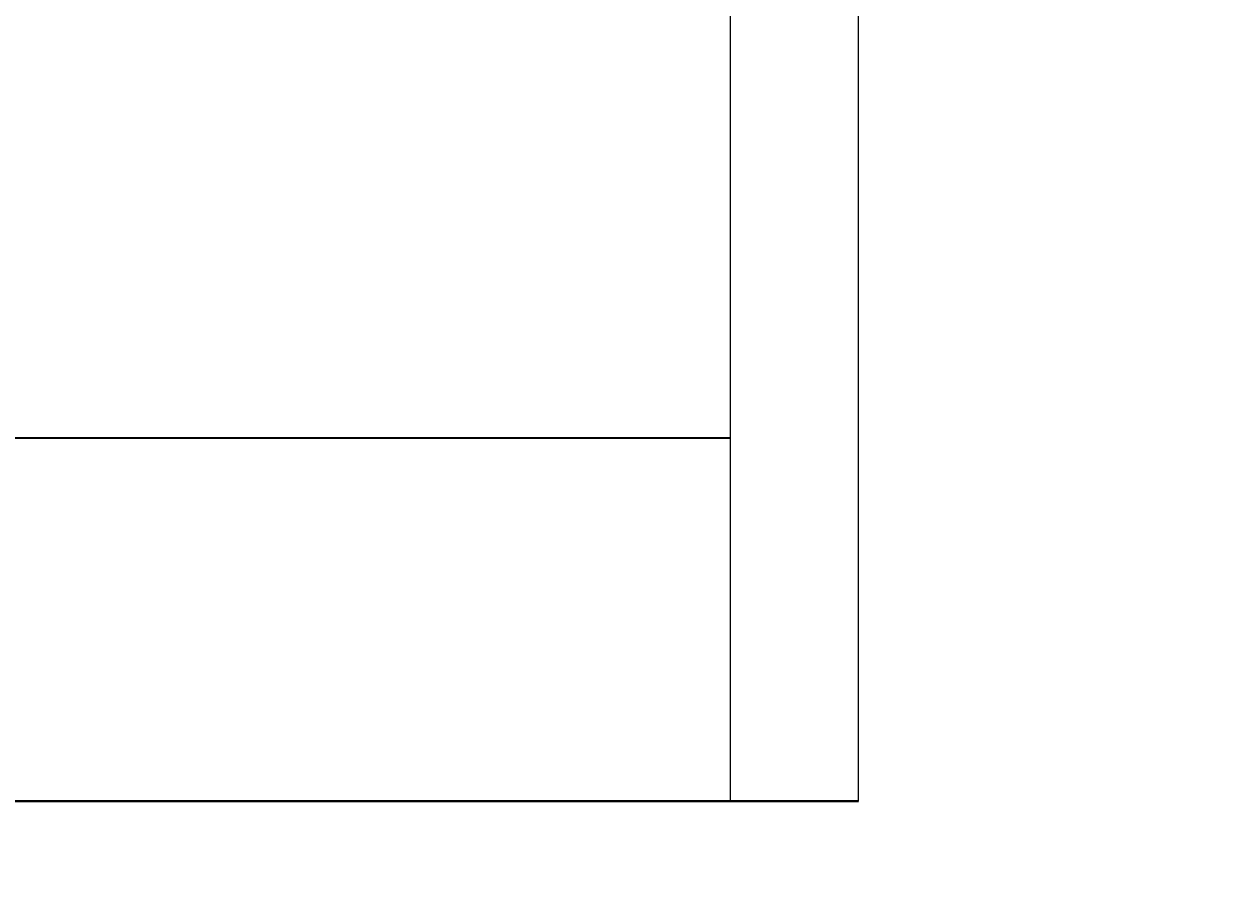
# Model space of a CAD drawing. Units: millimetres. Extents: x 19292 to 100733, y 12374 to 26974.
# Tile 5 of 24: x 29028 to 29777, y 14845 to 15391. Entities that reach past the tile are written whole.
import ezdxf

# ---------------------------------------------------------------- set-up
doc = ezdxf.new("R2010")
doc.units = ezdxf.units.MM
for name, color, linetype, lineweight in [('A-ANNO-DIMS', 2, 'Continuous', 18), ('A-DOOR', 4, 'Continuous', 25), ('A-FLOR-PATT', 252, 'Continuous', 13), ('A-WALL', 7, 'Continuous', 35)]:
    doc.layers.add(name, color=color, linetype=linetype, lineweight=lineweight)
doc.styles.get("Standard").update_dxf_attribs({"font": 'arial.ttf'})
doc.dimstyles.get("Standard").update_dxf_attribs({"dimtxt": 0.18, "dimasz": 0.18, "dimexe": 0.18, "dimexo": 0.0625, "dimgap": 0.09, "dimtad": 0, "dimtih": 1, "dimtoh": 1, "dimdec": 4, "dimzin": 0, "dimdsep": 46, "dimtxsty": 'Standard', "dimcen": 0.09, "dimadec": 0, "dimazin": 0, "dimtfac": 1, "dimtdec": 4, "dimtofl": 0, "dimtmove": 0, "dimatfit": 3, "dimfxl": 1, "dimtolj": 1, "dimtzin": 0, "dimarcsym": 0})

# ---------------------------------------------------------------- blocks, each defined once
blk = doc.blocks.new('*D79')
at = {"layer": 'A-ANNO-DIMS', "color": 0, "lineweight": -2, "transparency": 16777216}
for p, q in [((22694.13, 22860.66), (22694.13, 12808.81)), ((36144.17, 15985.66), (36144.17, 12808.81)), ((22694.31, 12808.99), (29418.73, 12808.99)), ((36143.99, 12808.99), (29419.57, 12808.99))]:
    blk.add_line(p, q, dxfattribs=at)
at = {"layer": 'A-ANNO-DIMS', "color": 0, "transparency": 16777216}
for points in [[(22694.31, 12809.02), (22694.31, 12808.96), (22694.13, 12808.99)], [(36143.99, 12809.02), (36143.99, 12808.96), (36144.17, 12808.99)]]:
    blk.add_solid(points, dxfattribs=at)
at = {"layer": 'Defpoints', "color": 0, "transparency": 16777216}
for p in [(22694.13, 22860.72), (36144.17, 15985.72), (36144.17, 12808.99)]:
    blk.add_point(p, dxfattribs=at)
at = {"layer": 'A-ANNO-DIMS', "color": 0, "transparency": 16777216, "insert": (29419.15, 12808.99), "char_height": 0.18, "attachment_point": 5}
blk.add_mtext('\\A1;13450', dxfattribs=at)
blk = doc.blocks.new('*D82')
at = {"layer": 'A-ANNO-DIMS', "color": 0, "lineweight": -2, "transparency": 16777216}
for p, q in [((27198.81, 13562.81), (27198.81, 23555.9)), ((27198.99, 23555.72), (29296.44, 23555.72)), ((31394.62, 23555.72), (29297.17, 23555.72)), ((31394.8, 13544.06), (31394.8, 23555.9))]:
    blk.add_line(p, q, dxfattribs=at)
at = {"layer": 'A-ANNO-DIMS', "color": 0, "transparency": 16777216}
for points in [[(27198.99, 23555.75), (27198.99, 23555.69), (27198.81, 23555.72)], [(31394.62, 23555.75), (31394.62, 23555.69), (31394.8, 23555.72)]]:
    blk.add_solid(points, dxfattribs=at)
at = {"layer": 'Defpoints', "color": 0, "transparency": 16777216}
for p in [(31394.8, 23555.72), (27198.81, 13562.75), (31394.8, 13543.99)]:
    blk.add_point(p, dxfattribs=at)
at = {"layer": 'A-ANNO-DIMS', "color": 0, "transparency": 16777216, "insert": (29296.81, 23555.72), "char_height": 0.18, "attachment_point": 5}
blk.add_mtext('\\A1;4196', dxfattribs=at)
blk = doc.blocks.new('*D86')
at = {"layer": 'A-ANNO-DIMS', "color": 0, "lineweight": -2, "transparency": 16777216}
for p, q in [((27198.81, 15132.81), (27198.81, 23555.9)), ((27198.99, 23555.72), (29198.45, 23555.72)), ((31198.63, 23555.72), (29199.18, 23555.72)), ((31198.81, 15132.81), (31198.81, 23555.9))]:
    blk.add_line(p, q, dxfattribs=at)
at = {"layer": 'A-ANNO-DIMS', "color": 0, "transparency": 16777216}
for points in [[(27198.99, 23555.75), (27198.99, 23555.69), (27198.81, 23555.72)], [(31198.63, 23555.75), (31198.63, 23555.69), (31198.81, 23555.72)]]:
    blk.add_solid(points, dxfattribs=at)
at = {"layer": 'Defpoints', "color": 0, "transparency": 16777216}
for p in [(31198.81, 23555.72), (27198.81, 15132.75), (31198.81, 15132.75)]:
    blk.add_point(p, dxfattribs=at)
at = {"layer": 'A-ANNO-DIMS', "color": 0, "transparency": 16777216, "insert": (29198.81, 23555.72), "char_height": 0.18, "attachment_point": 5}
blk.add_mtext('\\A1;4000', dxfattribs=at)

msp = doc.modelspace()

# ---------------------------------------------------------------- hatches: boundary and pattern name
at = {"layer": 'A-FLOR-PATT'}
h = msp.add_hatch(dxfattribs=at)
h.set_pattern_fill('CROSS', color=256, scale=40)
h.paths.add_polyline_path([(31394.799, 14906.403), (31051.542, 14906.403), (29468.571, 14906.403), (27198.815, 14906.403), (27198.815, 13543.993), (31394.799, 13543.993)])
h.paths.add_polyline_path([(27828.096, 14036.581), (30629.164, 14036.581), (30629.164, 14443.478), (27828.096, 14443.478)], flags=24)

# ---------------------------------------------------------------- linework, layer by layer
at = {"layer": 'A-DOOR'}
for p, q in [((29468.571, 14906.403), (29468.571, 15641.675)), ((29548.571, 14906.403), (29548.571, 15641.675)), ((29468.571, 14906.403), (29548.571, 14906.403)), ((29468.571, 14906.403), (29548.571, 14906.403))]:
    msp.add_line(p, q, dxfattribs=at)
msp.add_arc((29468.571, 14906.403), 735.272, 0, 90, dxfattribs=at)
at = {"layer": 'A-WALL'}
for points in [[(29548.571, 14906.403), (27198.815, 14906.403), (27198.815, 13562.748), (23348.815, 13562.748), (23348.815, 19010.725), (22694.132, 19010.725), (22694.132, 22860.725), (28369.132, 22860.725), (28369.132, 21460.725), (31169.132, 21460.725), (31169.132, 22460.725), (34419.132, 22460.725), (34419.132, 22208.026)], [(29468.571, 15132.748), (27198.815, 15132.748), (27198.815, 17812.748)], [(31051.542, 14906.403), (31394.799, 14906.403), (31394.799, 13543.993), (27198.815, 13543.993), (27198.815, 14906.403), (29548.571, 14906.403)]]:
    msp.add_lwpolyline(points, dxfattribs=at)

# ---------------------------------------------------------------- dimensions: what is measured, and where the dimension line sits
at = {"layer": 'A-ANNO-DIMS'}
for base, p1, p2, picture, middle in [((31394.799, 23555.725), (27198.815, 13562.748), (31394.799, 13543.993), '*D82', (29296.807, 23555.725)), ((31198.815, 23555.725), (27198.815, 15132.748), (31198.815, 15132.748), '*D86', (29198.815, 23555.725)), ((36144.169, 12808.993), (22694.132, 22860.725), (36144.169, 15985.725), '*D79', (29419.151, 12808.993))]:
    dim = msp.add_linear_dim(base=base, p1=p1, p2=p2, dimstyle='Standard', override={"dimdec": 0, "dimlfac": 1, "dimrnd": 0, "dimzin": 0, "dimdsep": 46, "dimlunit": 2}, dxfattribs=at)
    dim.commit()
    dim.dimension.update_dxf_attribs({"geometry": picture, "text_midpoint": middle})

doc.saveas('drawing.dxf')
